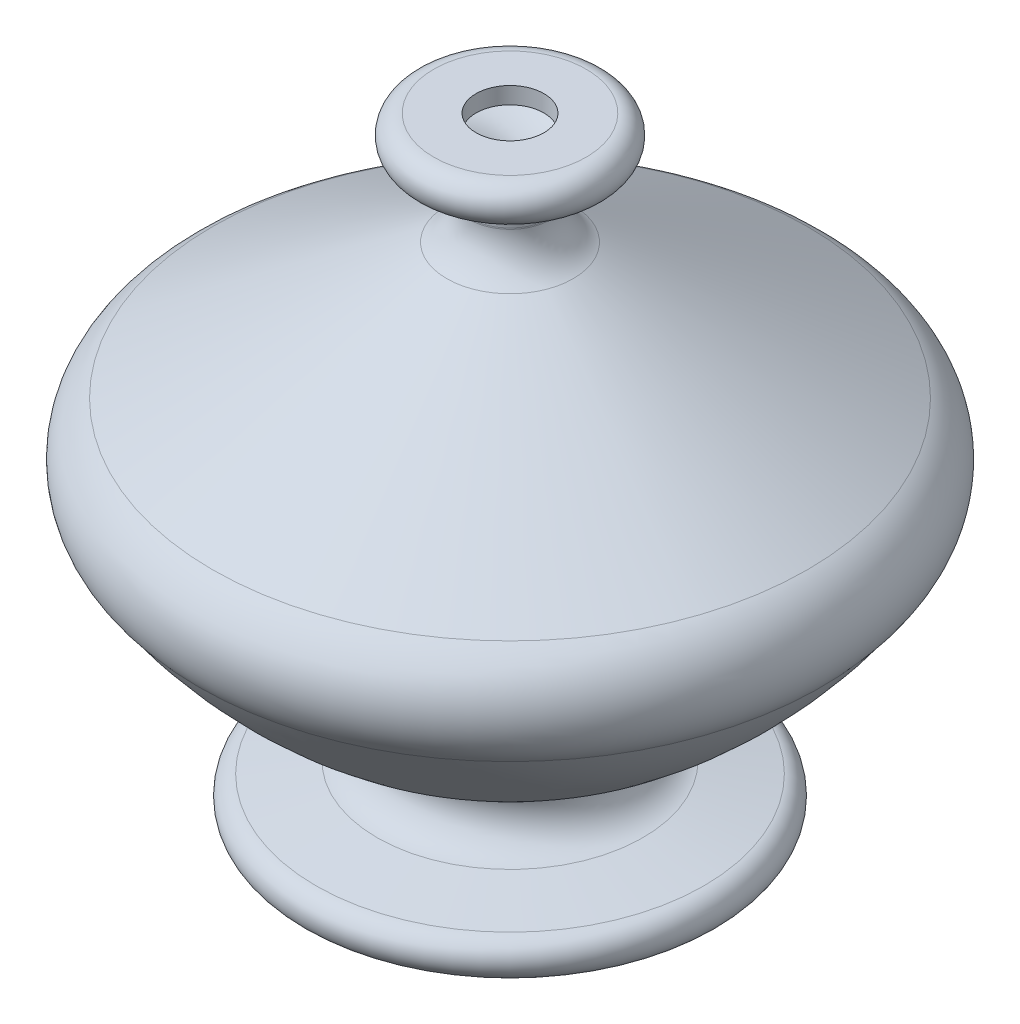
ISO-10303-21;
HEADER;
FILE_DESCRIPTION(('STEP AP214'),'2;1');
FILE_NAME('part.step','',(''),(''),'','','');
FILE_SCHEMA(('AUTOMOTIVE_DESIGN { 1 0 10303 214 1 1 1 1 }'));
ENDSEC;
DATA;
#1=APPLICATION_CONTEXT('core data for automotive mechanical design processes');
#2=APPLICATION_PROTOCOL_DEFINITION('international standard','automotive_design',2000,#1);
#3=PRODUCT_CONTEXT('',#1,'mechanical');
#4=PRODUCT('Part','Part','',(#3));
#5=PRODUCT_RELATED_PRODUCT_CATEGORY('part','',(#4));
#6=PRODUCT_DEFINITION_FORMATION('','',#4);
#7=PRODUCT_DEFINITION_CONTEXT('part definition',#1,'design');
#8=PRODUCT_DEFINITION('design','',#6,#7);
#9=PRODUCT_DEFINITION_SHAPE('','',#8);
#10=(LENGTH_UNIT() NAMED_UNIT(*) SI_UNIT(.MILLI.,.METRE.));
#11=(NAMED_UNIT(*) PLANE_ANGLE_UNIT() SI_UNIT($,.RADIAN.));
#12=(NAMED_UNIT(*) SI_UNIT($,.STERADIAN.) SOLID_ANGLE_UNIT());
#13=UNCERTAINTY_MEASURE_WITH_UNIT(LENGTH_MEASURE(1.E-05),#10,'distance_accuracy_value','');
#14=(GEOMETRIC_REPRESENTATION_CONTEXT(3) GLOBAL_UNCERTAINTY_ASSIGNED_CONTEXT((#13)) GLOBAL_UNIT_ASSIGNED_CONTEXT((#10,
#11,#12)) REPRESENTATION_CONTEXT('',''));
#15=CARTESIAN_POINT('',(0.,0.,0.));
#16=DIRECTION('',(0.,0.,1.));
#17=DIRECTION('',(1.,0.,0.));
#18=AXIS2_PLACEMENT_3D('',#15,#16,#17);
#19=CARTESIAN_POINT('',(0.,4.4,0.));
#20=DIRECTION('',(0.,1.,0.));
#21=DIRECTION('',(0.,0.,1.));
#22=AXIS2_PLACEMENT_3D('',#19,#20,#21);
#23=PLANE('',#22);
#24=CARTESIAN_POINT('',(0.,4.39999999999999,0.));
#25=DIRECTION('',(0.,1.,0.));
#26=DIRECTION('',(0.,0.,1.));
#27=AXIS2_PLACEMENT_3D('',#24,#25,#26);
#28=CIRCLE('',#27,50.);
#29=CARTESIAN_POINT('',(0.,4.39999999999999,50.));
#30=VERTEX_POINT('',#29);
#31=EDGE_CURVE('E10',#30,#30,#28,.T.);
#32=ORIENTED_EDGE('',*,*,#31,.T.);
#33=EDGE_LOOP('',(#32));
#34=FACE_BOUND('',#33,.T.);
#35=ADVANCED_FACE('F40',(#34),#23,.T.);
#36=CARTESIAN_POINT('',(0.,4.99999999999999,0.));
#37=DIRECTION('',(0.,1.,0.));
#38=DIRECTION('',(0.,0.,1.));
#39=AXIS2_PLACEMENT_3D('',#36,#37,#38);
#40=TOROIDAL_SURFACE('',#39,50.,0.599999999999995);
#41=CARTESIAN_POINT('',(0.,5.59021831279544,0.));
#42=DIRECTION('',(0.,1.,0.));
#43=DIRECTION('',(0.,0.,1.));
#44=AXIS2_PLACEMENT_3D('',#41,#42,#43);
#45=CIRCLE('',#44,50.1078996906432);
#46=CARTESIAN_POINT('',(0.,5.59021831279544,50.1078996906432));
#47=VERTEX_POINT('',#46);
#48=EDGE_CURVE('E43',#47,#47,#45,.T.);
#49=ORIENTED_EDGE('',*,*,#48,.T.);
#50=EDGE_LOOP('',(#49));
#51=FACE_BOUND('',#50,.T.);
#52=ORIENTED_EDGE('',*,*,#31,.F.);
#53=EDGE_LOOP('',(#52));
#54=FACE_BOUND('',#53,.T.);
#55=ADVANCED_FACE('F133',(#51,#54),#40,.F.);
#56=CARTESIAN_POINT('',(0.,5.59021831279544,0.));
#57=DIRECTION('',(0.,-1.,0.));
#58=DIRECTION('',(0.,0.,-1.));
#59=AXIS2_PLACEMENT_3D('',#56,#57,#58);
#60=CONICAL_SURFACE('',#59,50.1078996906432,1.38997983116206);
#61=CARTESIAN_POINT('',(0.,8.5184576809019,0.));
#62=DIRECTION('',(0.,1.,0.));
#63=DIRECTION('',(0.,0.,1.));
#64=AXIS2_PLACEMENT_3D('',#61,#62,#63);
#65=CIRCLE('',#64,34.0902402423009);
#66=CARTESIAN_POINT('',(0.,8.5184576809019,34.0902402423009));
#67=VERTEX_POINT('',#66);
#68=EDGE_CURVE('E50',#67,#67,#65,.T.);
#69=ORIENTED_EDGE('',*,*,#68,.T.);
#70=EDGE_LOOP('',(#69));
#71=FACE_BOUND('',#70,.T.);
#72=ORIENTED_EDGE('',*,*,#48,.F.);
#73=EDGE_LOOP('',(#72));
#74=FACE_BOUND('',#73,.T.);
#75=ADVANCED_FACE('F137',(#71,#74),#60,.F.);
#76=CARTESIAN_POINT('',(0.,21.7,0.));
#77=DIRECTION('',(0.,1.,0.));
#78=DIRECTION('',(0.,0.,1.));
#79=AXIS2_PLACEMENT_3D('',#76,#77,#78);
#80=TOROIDAL_SURFACE('',#79,36.5,13.4);
#81=CARTESIAN_POINT('',(0.,35.0477430693787,0.));
#82=DIRECTION('',(0.,1.,0.));
#83=DIRECTION('',(0.,0.,1.));
#84=AXIS2_PLACEMENT_3D('',#81,#82,#83);
#85=CIRCLE('',#84,35.3177331291744);
#86=CARTESIAN_POINT('',(0.,35.0477430693787,35.3177331291744));
#87=VERTEX_POINT('',#86);
#88=EDGE_CURVE('E51',#87,#87,#85,.T.);
#89=ORIENTED_EDGE('',*,*,#88,.T.);
#90=EDGE_LOOP('',(#89));
#91=FACE_BOUND('',#90,.T.);
#92=ORIENTED_EDGE('',*,*,#68,.F.);
#93=EDGE_LOOP('',(#92));
#94=FACE_BOUND('',#93,.T.);
#95=ADVANCED_FACE('F141',(#91,#94),#80,.T.);
#96=CARTESIAN_POINT('',(0.,141.481035556189,0.));
#97=DIRECTION('',(0.,1.,0.));
#98=DIRECTION('',(0.,0.,1.));
#99=AXIS2_PLACEMENT_3D('',#96,#97,#98);
#100=DEGENERATE_TOROIDAL_SURFACE('',#99,20.968270907506,120.4,.F.);
#101=CARTESIAN_POINT('',(0.,73.1766344230635,0.));
#102=DIRECTION('',(0.,1.,0.));
#103=DIRECTION('',(0.,0.,1.));
#104=AXIS2_PLACEMENT_3D('',#101,#102,#103);
#105=CIRCLE('',#104,78.1814582189275);
#106=CARTESIAN_POINT('',(0.,73.1766344230635,78.1814582189275));
#107=VERTEX_POINT('',#106);
#108=EDGE_CURVE('E57',#107,#107,#105,.T.);
#109=ORIENTED_EDGE('',*,*,#108,.T.);
#110=EDGE_LOOP('',(#109));
#111=FACE_BOUND('',#110,.T.);
#112=ORIENTED_EDGE('',*,*,#88,.F.);
#113=EDGE_LOOP('',(#112));
#114=FACE_BOUND('',#113,.T.);
#115=ADVANCED_FACE('F147',(#111,#114),#100,.T.);
#116=CARTESIAN_POINT('',(0.,81.4,0.));
#117=DIRECTION('',(0.,1.,0.));
#118=DIRECTION('',(0.,0.,1.));
#119=AXIS2_PLACEMENT_3D('',#116,#117,#118);
#120=TOROIDAL_SURFACE('',#119,70.,11.6);
#121=CARTESIAN_POINT('',(0.,91.4458946838995,0.));
#122=DIRECTION('',(0.,1.,0.));
#123=DIRECTION('',(0.,0.,1.));
#124=AXIS2_PLACEMENT_3D('',#121,#122,#123);
#125=CIRCLE('',#124,75.8000000000001);
#126=CARTESIAN_POINT('',(0.,91.4458946838994,-75.8000000000001));
#127=VERTEX_POINT('',#126);
#128=EDGE_CURVE('E56',#127,#127,#125,.T.);
#129=ORIENTED_EDGE('',*,*,#128,.T.);
#130=EDGE_LOOP('',(#129));
#131=FACE_BOUND('',#130,.T.);
#132=ORIENTED_EDGE('',*,*,#108,.F.);
#133=EDGE_LOOP('',(#132));
#134=FACE_BOUND('',#133,.T.);
#135=ADVANCED_FACE('F152',(#131,#134),#120,.F.);
#136=CARTESIAN_POINT('',(0.,91.4458946838995,0.));
#137=DIRECTION('',(0.,-1.,0.));
#138=DIRECTION('',(0.,0.,-1.));
#139=AXIS2_PLACEMENT_3D('',#136,#137,#138);
#140=CONICAL_SURFACE('',#139,75.8000000000001,1.04719755119659);
#141=CARTESIAN_POINT('',(0.,126.895201212143,0.));
#142=DIRECTION('',(0.,1.,0.));
#143=DIRECTION('',(0.,0.,1.));
#144=AXIS2_PLACEMENT_3D('',#141,#142,#143);
#145=CIRCLE('',#144,14.3999999999999);
#146=CARTESIAN_POINT('',(0.,126.895201212143,-14.4));
#147=VERTEX_POINT('',#146);
#148=EDGE_CURVE('E65',#147,#147,#145,.T.);
#149=CARTESIAN_POINT('',(0.,126.895201212143,-14.4));
#150=CARTESIAN_POINT('',(0.,126.525937602474,-15.0395833333333));
#151=CARTESIAN_POINT('',(0.,126.156673992805,-15.6791666666666));
#152=CARTESIAN_POINT('',(0.,125.418146773466,-16.9583333333333));
#153=CARTESIAN_POINT('',(0.,125.048883163797,-17.5979166666666));
#154=CARTESIAN_POINT('',(0.,124.310355944459,-18.8770833333333));
#155=CARTESIAN_POINT('',(0.,123.941092334789,-19.5166666666666));
#156=CARTESIAN_POINT('',(0.,123.202565115451,-20.7958333333333));
#157=CARTESIAN_POINT('',(0.,122.833301505782,-21.4354166666666));
#158=CARTESIAN_POINT('',(0.,122.094774286443,-22.7145833333333));
#159=CARTESIAN_POINT('',(0.,121.725510676774,-23.3541666666666));
#160=CARTESIAN_POINT('',(0.,120.986983457436,-24.6333333333333));
#161=CARTESIAN_POINT('',(0.,120.617719847767,-25.2729166666666));
#162=CARTESIAN_POINT('',(0.,119.879192628428,-26.5520833333333));
#163=CARTESIAN_POINT('',(0.,119.509929018759,-27.1916666666666));
#164=CARTESIAN_POINT('',(0.,118.771401799421,-28.4708333333333));
#165=CARTESIAN_POINT('',(0.,118.402138189751,-29.1104166666666));
#166=CARTESIAN_POINT('',(0.,117.663610970413,-30.3895833333333));
#167=CARTESIAN_POINT('',(0.,117.294347360744,-31.0291666666666));
#168=CARTESIAN_POINT('',(0.,116.555820141405,-32.3083333333333));
#169=CARTESIAN_POINT('',(0.,116.186556531736,-32.9479166666667));
#170=CARTESIAN_POINT('',(0.,115.448029312398,-34.2270833333333));
#171=CARTESIAN_POINT('',(0.,115.078765702728,-34.8666666666667));
#172=CARTESIAN_POINT('',(0.,114.34023848339,-36.1458333333333));
#173=CARTESIAN_POINT('',(0.,113.970974873721,-36.7854166666667));
#174=CARTESIAN_POINT('',(0.,113.232447654382,-38.0645833333333));
#175=CARTESIAN_POINT('',(0.,112.863184044713,-38.7041666666667));
#176=CARTESIAN_POINT('',(0.,112.124656825375,-39.9833333333333));
#177=CARTESIAN_POINT('',(0.,111.755393215706,-40.6229166666667));
#178=CARTESIAN_POINT('',(0.,111.016865996367,-41.9020833333333));
#179=CARTESIAN_POINT('',(0.,110.647602386698,-42.5416666666667));
#180=CARTESIAN_POINT('',(0.,109.90907516736,-43.8208333333333));
#181=CARTESIAN_POINT('',(0.,109.53981155769,-44.4604166666667));
#182=CARTESIAN_POINT('',(0.,108.801284338352,-45.7395833333333));
#183=CARTESIAN_POINT('',(0.,108.432020728683,-46.3791666666667));
#184=CARTESIAN_POINT('',(0.,107.693493509344,-47.6583333333333));
#185=CARTESIAN_POINT('',(0.,107.324229899675,-48.2979166666667));
#186=CARTESIAN_POINT('',(0.,106.585702680337,-49.5770833333333));
#187=CARTESIAN_POINT('',(0.,106.216439070668,-50.2166666666667));
#188=CARTESIAN_POINT('',(0.,105.477911851329,-51.4958333333334));
#189=CARTESIAN_POINT('',(0.,105.10864824166,-52.1354166666667));
#190=CARTESIAN_POINT('',(0.,104.370121022322,-53.4145833333334));
#191=CARTESIAN_POINT('',(0.,104.000857412652,-54.0541666666667));
#192=CARTESIAN_POINT('',(0.,103.262330193314,-55.3333333333334));
#193=CARTESIAN_POINT('',(0.,102.893066583645,-55.9729166666667));
#194=CARTESIAN_POINT('',(0.,102.154539364306,-57.2520833333334));
#195=CARTESIAN_POINT('',(0.,101.785275754637,-57.8916666666667));
#196=CARTESIAN_POINT('',(0.,101.046748535299,-59.1708333333334));
#197=CARTESIAN_POINT('',(0.,100.67748492563,-59.8104166666667));
#198=CARTESIAN_POINT('',(0.,99.9389577062911,-61.0895833333334));
#199=CARTESIAN_POINT('',(0.,99.5696940966219,-61.7291666666667));
#200=CARTESIAN_POINT('',(0.,98.8311668772835,-63.0083333333334));
#201=CARTESIAN_POINT('',(0.,98.4619032676143,-63.6479166666667));
#202=CARTESIAN_POINT('',(0.,97.7233760482759,-64.9270833333334));
#203=CARTESIAN_POINT('',(0.,97.3541124386067,-65.5666666666667));
#204=CARTESIAN_POINT('',(0.,96.6155852192683,-66.8458333333334));
#205=CARTESIAN_POINT('',(0.,96.2463216095991,-67.4854166666667));
#206=CARTESIAN_POINT('',(0.,95.5077943902607,-68.7645833333334));
#207=CARTESIAN_POINT('',(0.,95.1385307805915,-69.4041666666667));
#208=CARTESIAN_POINT('',(0.,94.4000035612531,-70.6833333333334));
#209=CARTESIAN_POINT('',(0.,94.0307399515839,-71.3229166666667));
#210=CARTESIAN_POINT('',(0.,93.2922127322455,-72.6020833333334));
#211=CARTESIAN_POINT('',(0.,92.9229491225762,-73.2416666666667));
#212=CARTESIAN_POINT('',(0.,92.1844219032378,-74.5208333333334));
#213=CARTESIAN_POINT('',(0.,91.8151582935686,-75.1604166666667));
#214=CARTESIAN_POINT('',(0.,91.4458946838994,-75.8000000000001));
#215=B_SPLINE_CURVE_WITH_KNOTS('',3,(#149,#150,#151,#152,#153,#154,#155,#156,#157,#158,#159,
#160,#161,#162,#163,#164,#165,#166,#167,#168,#169,#170,#171,#172,#173,#174,#175,#176,#177,#178,
#179,#180,#181,#182,#183,#184,#185,#186,#187,#188,#189,#190,#191,#192,#193,#194,#195,#196,#197,
#198,#199,#200,#201,#202,#203,#204,#205,#206,#207,#208,#209,#210,#211,#212,#213,#214),
.UNSPECIFIED.,.F.,.F.,(4,2,2,2,2,2,2,2,2,2,2,2,2,2,2,2,2,2,2,2,2,2,2,2,2,2,2,2,2,2,2,2,4),(0.,
2.21558165801521,4.43116331603041,6.64674497404561,8.86232663206081,11.077908290076,
13.2934899480912,15.5090716061064,17.7246532641216,19.9402349221368,22.155816580152,
24.3713982381672,26.5869798961824,28.8025615541976,31.0181432122128,33.233724870228,
35.4493065282432,37.6648881862584,39.8804698442736,42.0960515022888,44.311633160304,
46.5272148183192,48.7427964763344,50.9583781343496,53.1739597923648,55.38954145038,
57.6051231083952,59.8207047664104,62.0362864244256,64.2518680824408,66.467449740456,
68.6830313984712,70.8986130564864),.UNSPECIFIED.);
#216=EDGE_CURVE('BSEAM158',#147,#127,#215,.T.);
#217=ORIENTED_EDGE('',*,*,#148,.T.);
#218=ORIENTED_EDGE('',*,*,#128,.F.);
#219=ORIENTED_EDGE('',*,*,#216,.T.);
#220=ORIENTED_EDGE('',*,*,#216,.F.);
#221=EDGE_LOOP('',(#217,#219,#218,#220));
#222=FACE_BOUND('',#221,.T.);
#223=ADVANCED_FACE('F158',(#222),#140,.F.);
#224=CARTESIAN_POINT('',(0.,141.098017834208,0.));
#225=DIRECTION('',(0.,1.,0.));
#226=DIRECTION('',(0.,0.,1.));
#227=AXIS2_PLACEMENT_3D('',#224,#225,#226);
#228=TOROIDAL_SURFACE('',#227,22.6,16.4);
#229=CARTESIAN_POINT('',(0.,141.098017834208,0.));
#230=DIRECTION('',(0.,1.,0.));
#231=DIRECTION('',(0.,0.,1.));
#232=AXIS2_PLACEMENT_3D('',#229,#230,#231);
#233=CIRCLE('',#232,6.2);
#234=CARTESIAN_POINT('',(0.,141.098017834208,6.2));
#235=VERTEX_POINT('',#234);
#236=EDGE_CURVE('E63',#235,#235,#233,.T.);
#237=ORIENTED_EDGE('',*,*,#236,.T.);
#238=EDGE_LOOP('',(#237));
#239=FACE_BOUND('',#238,.T.);
#240=ORIENTED_EDGE('',*,*,#148,.F.);
#241=EDGE_LOOP('',(#240));
#242=FACE_BOUND('',#241,.T.);
#243=ADVANCED_FACE('F165',(#239,#242),#228,.T.);
#244=CARTESIAN_POINT('',(0.,194.540686073728,0.));
#245=DIRECTION('',(0.,1.,0.));
#246=DIRECTION('',(0.,0.,1.));
#247=AXIS2_PLACEMENT_3D('',#244,#245,#246);
#248=CYLINDRICAL_SURFACE('',#247,6.2);
#249=CARTESIAN_POINT('',(0.,141.403935941769,0.));
#250=DIRECTION('',(0.,1.,0.));
#251=DIRECTION('',(0.,0.,1.));
#252=AXIS2_PLACEMENT_3D('',#249,#250,#251);
#253=CIRCLE('',#252,6.19999999999999);
#254=CARTESIAN_POINT('',(0.,141.403935941769,6.19999999999999));
#255=VERTEX_POINT('',#254);
#256=EDGE_CURVE('E68',#255,#255,#253,.T.);
#257=ORIENTED_EDGE('',*,*,#256,.T.);
#258=EDGE_LOOP('',(#257));
#259=FACE_BOUND('',#258,.T.);
#260=ORIENTED_EDGE('',*,*,#236,.F.);
#261=EDGE_LOOP('',(#260));
#262=FACE_BOUND('',#261,.T.);
#263=ADVANCED_FACE('F167',(#259,#262),#248,.F.);
#264=CARTESIAN_POINT('',(0.,141.403935941769,0.));
#265=DIRECTION('',(0.,1.,0.));
#266=DIRECTION('',(0.,0.,1.));
#267=AXIS2_PLACEMENT_3D('',#264,#265,#266);
#268=TOROIDAL_SURFACE('',#267,18.6,12.4);
#269=CARTESIAN_POINT('',(0.,153.5281168675,0.));
#270=DIRECTION('',(0.,1.,0.));
#271=DIRECTION('',(0.,0.,1.));
#272=AXIS2_PLACEMENT_3D('',#269,#270,#271);
#273=CIRCLE('',#272,15.9991853429861);
#274=CARTESIAN_POINT('',(0.,153.5281168675,15.9991853429861));
#275=VERTEX_POINT('',#274);
#276=EDGE_CURVE('E72',#275,#275,#273,.T.);
#277=ORIENTED_EDGE('',*,*,#276,.T.);
#278=EDGE_LOOP('',(#277));
#279=FACE_BOUND('',#278,.T.);
#280=ORIENTED_EDGE('',*,*,#256,.F.);
#281=EDGE_LOOP('',(#280));
#282=FACE_BOUND('',#281,.T.);
#283=ADVANCED_FACE('F168',(#279,#282),#268,.T.);
#284=CARTESIAN_POINT('',(0.,153.5281168675,0.));
#285=DIRECTION('',(0.,1.,0.));
#286=DIRECTION('',(0.,0.,1.));
#287=AXIS2_PLACEMENT_3D('',#284,#285,#286);
#288=CONICAL_SURFACE('',#287,15.9991853429861,1.35948410089142);
#289=CARTESIAN_POINT('',(0.,154.413346084239,0.));
#290=DIRECTION('',(0.,1.,0.));
#291=DIRECTION('',(0.,0.,1.));
#292=AXIS2_PLACEMENT_3D('',#289,#290,#291);
#293=CIRCLE('',#292,20.1258458705007);
#294=CARTESIAN_POINT('',(0.,154.413346084239,20.1258458705007));
#295=VERTEX_POINT('',#294);
#296=EDGE_CURVE('E74',#295,#295,#293,.T.);
#297=ORIENTED_EDGE('',*,*,#296,.T.);
#298=EDGE_LOOP('',(#297));
#299=FACE_BOUND('',#298,.T.);
#300=ORIENTED_EDGE('',*,*,#276,.F.);
#301=EDGE_LOOP('',(#300));
#302=FACE_BOUND('',#301,.T.);
#303=ADVANCED_FACE('F171',(#299,#302),#288,.F.);
#304=CARTESIAN_POINT('',(0.,155.,0.));
#305=DIRECTION('',(0.,1.,0.));
#306=DIRECTION('',(0.,0.,1.));
#307=AXIS2_PLACEMENT_3D('',#304,#305,#306);
#308=TOROIDAL_SURFACE('',#307,20.,0.599999999999995);
#309=CARTESIAN_POINT('',(0.,155.6,0.));
#310=DIRECTION('',(0.,1.,0.));
#311=DIRECTION('',(0.,0.,1.));
#312=AXIS2_PLACEMENT_3D('',#309,#310,#311);
#313=CIRCLE('',#312,20.);
#314=CARTESIAN_POINT('',(0.,155.6,20.));
#315=VERTEX_POINT('',#314);
#316=EDGE_CURVE('E80',#315,#315,#313,.T.);
#317=ORIENTED_EDGE('',*,*,#316,.T.);
#318=EDGE_LOOP('',(#317));
#319=FACE_BOUND('',#318,.T.);
#320=ORIENTED_EDGE('',*,*,#296,.F.);
#321=EDGE_LOOP('',(#320));
#322=FACE_BOUND('',#321,.T.);
#323=ADVANCED_FACE('F178',(#319,#322),#308,.F.);
#324=CARTESIAN_POINT('',(-20.,155.6,0.));
#325=DIRECTION('',(0.,-1.,0.));
#326=DIRECTION('',(0.,0.,-1.));
#327=AXIS2_PLACEMENT_3D('',#324,#325,#326);
#328=PLANE('',#327);
#329=CARTESIAN_POINT('',(0.,155.6,0.));
#330=DIRECTION('',(0.,1.,0.));
#331=DIRECTION('',(0.,0.,1.));
#332=AXIS2_PLACEMENT_3D('',#329,#330,#331);
#333=CIRCLE('',#332,8.9);
#334=CARTESIAN_POINT('',(0.,155.6,8.9));
#335=VERTEX_POINT('',#334);
#336=EDGE_CURVE('E78',#335,#335,#333,.T.);
#337=ORIENTED_EDGE('',*,*,#336,.T.);
#338=EDGE_LOOP('',(#337));
#339=FACE_BOUND('',#338,.T.);
#340=ORIENTED_EDGE('',*,*,#316,.F.);
#341=EDGE_LOOP('',(#340));
#342=FACE_BOUND('',#341,.T.);
#343=ADVANCED_FACE('F185',(#339,#342),#328,.T.);
#344=CARTESIAN_POINT('',(0.,194.540686073728,0.));
#345=DIRECTION('',(0.,1.,0.));
#346=DIRECTION('',(0.,0.,1.));
#347=AXIS2_PLACEMENT_3D('',#344,#345,#346);
#348=CYLINDRICAL_SURFACE('',#347,8.9);
#349=CARTESIAN_POINT('',(0.,160.,0.));
#350=DIRECTION('',(0.,1.,0.));
#351=DIRECTION('',(0.,0.,1.));
#352=AXIS2_PLACEMENT_3D('',#349,#350,#351);
#353=CIRCLE('',#352,8.9);
#354=CARTESIAN_POINT('',(0.,160.,8.9));
#355=VERTEX_POINT('',#354);
#356=EDGE_CURVE('E83',#355,#355,#353,.T.);
#357=ORIENTED_EDGE('',*,*,#356,.T.);
#358=EDGE_LOOP('',(#357));
#359=FACE_BOUND('',#358,.T.);
#360=ORIENTED_EDGE('',*,*,#336,.F.);
#361=EDGE_LOOP('',(#360));
#362=FACE_BOUND('',#361,.T.);
#363=ADVANCED_FACE('F187',(#359,#362),#348,.F.);
#364=CARTESIAN_POINT('',(-20.,160.,0.));
#365=DIRECTION('',(0.,1.,0.));
#366=DIRECTION('',(0.,0.,1.));
#367=AXIS2_PLACEMENT_3D('',#364,#365,#366);
#368=PLANE('',#367);
#369=CARTESIAN_POINT('',(0.,160.,0.));
#370=DIRECTION('',(0.,1.,0.));
#371=DIRECTION('',(0.,0.,1.));
#372=AXIS2_PLACEMENT_3D('',#369,#370,#371);
#373=CIRCLE('',#372,20.);
#374=CARTESIAN_POINT('',(0.,160.,20.));
#375=VERTEX_POINT('',#374);
#376=EDGE_CURVE('E88',#375,#375,#373,.T.);
#377=ORIENTED_EDGE('',*,*,#376,.T.);
#378=EDGE_LOOP('',(#377));
#379=FACE_BOUND('',#378,.T.);
#380=ORIENTED_EDGE('',*,*,#356,.F.);
#381=EDGE_LOOP('',(#380));
#382=FACE_BOUND('',#381,.T.);
#383=ADVANCED_FACE('F188',(#379,#382),#368,.T.);
#384=CARTESIAN_POINT('',(0.,155.,0.));
#385=DIRECTION('',(0.,1.,0.));
#386=DIRECTION('',(0.,0.,1.));
#387=AXIS2_PLACEMENT_3D('',#384,#385,#386);
#388=TOROIDAL_SURFACE('',#387,20.,4.99999999999999);
#389=CARTESIAN_POINT('',(0.,150.111217368657,0.));
#390=DIRECTION('',(0.,1.,0.));
#391=DIRECTION('',(0.,0.,1.));
#392=AXIS2_PLACEMENT_3D('',#389,#390,#391);
#393=CIRCLE('',#392,21.0487155875056);
#394=CARTESIAN_POINT('',(0.,150.111217368657,21.0487155875056));
#395=VERTEX_POINT('',#394);
#396=EDGE_CURVE('E90',#395,#395,#393,.T.);
#397=ORIENTED_EDGE('',*,*,#396,.T.);
#398=EDGE_LOOP('',(#397));
#399=FACE_BOUND('',#398,.T.);
#400=ORIENTED_EDGE('',*,*,#376,.F.);
#401=EDGE_LOOP('',(#400));
#402=FACE_BOUND('',#401,.T.);
#403=ADVANCED_FACE('F192',(#399,#402),#388,.T.);
#404=CARTESIAN_POINT('',(0.,150.111217368657,0.));
#405=DIRECTION('',(0.,1.,0.));
#406=DIRECTION('',(0.,0.,1.));
#407=AXIS2_PLACEMENT_3D('',#404,#405,#406);
#408=CONICAL_SURFACE('',#407,21.0487155875056,1.35948410089141);
#409=CARTESIAN_POINT('',(0.,149.225988151918,0.));
#410=DIRECTION('',(0.,1.,0.));
#411=DIRECTION('',(0.,0.,1.));
#412=AXIS2_PLACEMENT_3D('',#409,#410,#411);
#413=CIRCLE('',#412,16.922055059991);
#414=CARTESIAN_POINT('',(0.,149.225988151918,16.922055059991));
#415=VERTEX_POINT('',#414);
#416=EDGE_CURVE('E95',#415,#415,#413,.T.);
#417=ORIENTED_EDGE('',*,*,#416,.T.);
#418=EDGE_LOOP('',(#417));
#419=FACE_BOUND('',#418,.T.);
#420=ORIENTED_EDGE('',*,*,#396,.F.);
#421=EDGE_LOOP('',(#420));
#422=FACE_BOUND('',#421,.T.);
#423=ADVANCED_FACE('F196',(#419,#422),#408,.T.);
#424=CARTESIAN_POINT('',(0.,141.403935941769,0.));
#425=DIRECTION('',(0.,1.,0.));
#426=DIRECTION('',(0.,0.,1.));
#427=AXIS2_PLACEMENT_3D('',#424,#425,#426);
#428=TOROIDAL_SURFACE('',#427,18.6,8.00000000000001);
#429=CARTESIAN_POINT('',(0.,141.403935941769,0.));
#430=DIRECTION('',(0.,1.,0.));
#431=DIRECTION('',(0.,0.,1.));
#432=AXIS2_PLACEMENT_3D('',#429,#430,#431);
#433=CIRCLE('',#432,10.6);
#434=CARTESIAN_POINT('',(0.,141.403935941769,10.6));
#435=VERTEX_POINT('',#434);
#436=EDGE_CURVE('E92',#435,#435,#433,.T.);
#437=ORIENTED_EDGE('',*,*,#436,.T.);
#438=EDGE_LOOP('',(#437));
#439=FACE_BOUND('',#438,.T.);
#440=ORIENTED_EDGE('',*,*,#416,.F.);
#441=EDGE_LOOP('',(#440));
#442=FACE_BOUND('',#441,.T.);
#443=ADVANCED_FACE('F205',(#439,#442),#428,.F.);
#444=CARTESIAN_POINT('',(0.,194.540686073728,0.));
#445=DIRECTION('',(0.,1.,0.));
#446=DIRECTION('',(0.,0.,1.));
#447=AXIS2_PLACEMENT_3D('',#444,#445,#446);
#448=CYLINDRICAL_SURFACE('',#447,10.6);
#449=CARTESIAN_POINT('',(0.,141.098017834208,0.));
#450=DIRECTION('',(0.,1.,0.));
#451=DIRECTION('',(0.,0.,1.));
#452=AXIS2_PLACEMENT_3D('',#449,#450,#451);
#453=CIRCLE('',#452,10.6);
#454=CARTESIAN_POINT('',(0.,141.098017834208,10.6));
#455=VERTEX_POINT('',#454);
#456=EDGE_CURVE('E98',#455,#455,#453,.T.);
#457=ORIENTED_EDGE('',*,*,#456,.T.);
#458=EDGE_LOOP('',(#457));
#459=FACE_BOUND('',#458,.T.);
#460=ORIENTED_EDGE('',*,*,#436,.F.);
#461=EDGE_LOOP('',(#460));
#462=FACE_BOUND('',#461,.T.);
#463=ADVANCED_FACE('F206',(#459,#462),#448,.T.);
#464=CARTESIAN_POINT('',(0.,141.098017834208,0.));
#465=DIRECTION('',(0.,1.,0.));
#466=DIRECTION('',(0.,0.,1.));
#467=AXIS2_PLACEMENT_3D('',#464,#465,#466);
#468=TOROIDAL_SURFACE('',#467,22.6,12.);
#469=CARTESIAN_POINT('',(0.,130.705712988794,0.));
#470=DIRECTION('',(0.,1.,0.));
#471=DIRECTION('',(0.,0.,1.));
#472=AXIS2_PLACEMENT_3D('',#469,#470,#471);
#473=CIRCLE('',#472,16.5999999999999);
#474=CARTESIAN_POINT('',(0.,130.705712988794,-16.6));
#475=VERTEX_POINT('',#474);
#476=EDGE_CURVE('E101',#475,#475,#473,.T.);
#477=ORIENTED_EDGE('',*,*,#476,.T.);
#478=EDGE_LOOP('',(#477));
#479=FACE_BOUND('',#478,.T.);
#480=ORIENTED_EDGE('',*,*,#456,.F.);
#481=EDGE_LOOP('',(#480));
#482=FACE_BOUND('',#481,.T.);
#483=ADVANCED_FACE('F209',(#479,#482),#468,.F.);
#484=CARTESIAN_POINT('',(0.,130.705712988794,0.));
#485=DIRECTION('',(0.,-1.,0.));
#486=DIRECTION('',(0.,0.,-1.));
#487=AXIS2_PLACEMENT_3D('',#484,#485,#486);
#488=CONICAL_SURFACE('',#487,16.5999999999999,1.04719755119659);
#489=CARTESIAN_POINT('',(0.,95.256406460551,0.));
#490=DIRECTION('',(0.,1.,0.));
#491=DIRECTION('',(0.,0.,1.));
#492=AXIS2_PLACEMENT_3D('',#489,#490,#491);
#493=CIRCLE('',#492,78.0000000000001);
#494=CARTESIAN_POINT('',(0.,95.256406460551,-78.0000000000001));
#495=VERTEX_POINT('',#494);
#496=EDGE_CURVE('E102',#495,#495,#493,.T.);
#497=CARTESIAN_POINT('',(0.,95.256406460551,-78.0000000000001));
#498=CARTESIAN_POINT('',(0.,95.6256700702202,-77.3604166666667));
#499=CARTESIAN_POINT('',(0.,95.9949336798894,-76.7208333333334));
#500=CARTESIAN_POINT('',(0.,96.7334608992278,-75.4416666666667));
#501=CARTESIAN_POINT('',(0.,97.102724508897,-74.8020833333334));
#502=CARTESIAN_POINT('',(0.,97.8412517282354,-73.5229166666667));
#503=CARTESIAN_POINT('',(0.,98.2105153379046,-72.8833333333334));
#504=CARTESIAN_POINT('',(0.,98.949042557243,-71.6041666666667));
#505=CARTESIAN_POINT('',(0.,99.3183061669122,-70.9645833333334));
#506=CARTESIAN_POINT('',(0.,100.056833386251,-69.6854166666667));
#507=CARTESIAN_POINT('',(0.,100.42609699592,-69.0458333333334));
#508=CARTESIAN_POINT('',(0.,101.164624215258,-67.7666666666667));
#509=CARTESIAN_POINT('',(0.,101.533887824927,-67.1270833333334));
#510=CARTESIAN_POINT('',(0.,102.272415044266,-65.8479166666667));
#511=CARTESIAN_POINT('',(0.,102.641678653935,-65.2083333333334));
#512=CARTESIAN_POINT('',(0.,103.380205873273,-63.9291666666667));
#513=CARTESIAN_POINT('',(0.,103.749469482943,-63.2895833333334));
#514=CARTESIAN_POINT('',(0.,104.487996702281,-62.0104166666667));
#515=CARTESIAN_POINT('',(0.,104.85726031195,-61.3708333333334));
#516=CARTESIAN_POINT('',(0.,105.595787531289,-60.0916666666667));
#517=CARTESIAN_POINT('',(0.,105.965051140958,-59.4520833333334));
#518=CARTESIAN_POINT('',(0.,106.703578360296,-58.1729166666667));
#519=CARTESIAN_POINT('',(0.,107.072841969965,-57.5333333333334));
#520=CARTESIAN_POINT('',(0.,107.811369189304,-56.2541666666667));
#521=CARTESIAN_POINT('',(0.,108.180632798973,-55.6145833333334));
#522=CARTESIAN_POINT('',(0.,108.919160018311,-54.3354166666667));
#523=CARTESIAN_POINT('',(0.,109.288423627981,-53.6958333333334));
#524=CARTESIAN_POINT('',(0.,110.026950847319,-52.4166666666667));
#525=CARTESIAN_POINT('',(0.,110.396214456988,-51.7770833333334));
#526=CARTESIAN_POINT('',(0.,111.134741676327,-50.4979166666667));
#527=CARTESIAN_POINT('',(0.,111.504005285996,-49.8583333333334));
#528=CARTESIAN_POINT('',(0.,112.242532505334,-48.5791666666667));
#529=CARTESIAN_POINT('',(0.,112.611796115004,-47.9395833333334));
#530=CARTESIAN_POINT('',(0.,113.350323334342,-46.6604166666667));
#531=CARTESIAN_POINT('',(0.,113.719586944011,-46.0208333333333));
#532=CARTESIAN_POINT('',(0.,114.45811416335,-44.7416666666667));
#533=CARTESIAN_POINT('',(0.,114.827377773019,-44.1020833333333));
#534=CARTESIAN_POINT('',(0.,115.565904992357,-42.8229166666667));
#535=CARTESIAN_POINT('',(0.,115.935168602026,-42.1833333333334));
#536=CARTESIAN_POINT('',(0.,116.673695821365,-40.9041666666667));
#537=CARTESIAN_POINT('',(0.,117.042959431034,-40.2645833333333));
#538=CARTESIAN_POINT('',(0.,117.781486650372,-38.9854166666667));
#539=CARTESIAN_POINT('',(0.,118.150750260042,-38.3458333333333));
#540=CARTESIAN_POINT('',(0.,118.88927747938,-37.0666666666667));
#541=CARTESIAN_POINT('',(0.,119.258541089049,-36.4270833333333));
#542=CARTESIAN_POINT('',(0.,119.997068308388,-35.1479166666667));
#543=CARTESIAN_POINT('',(0.,120.366331918057,-34.5083333333333));
#544=CARTESIAN_POINT('',(0.,121.104859137395,-33.2291666666667));
#545=CARTESIAN_POINT('',(0.,121.474122747064,-32.5895833333333));
#546=CARTESIAN_POINT('',(0.,122.212649966403,-31.3104166666667));
#547=CARTESIAN_POINT('',(0.,122.581913576072,-30.6708333333333));
#548=CARTESIAN_POINT('',(0.,123.32044079541,-29.3916666666667));
#549=CARTESIAN_POINT('',(0.,123.68970440508,-28.7520833333333));
#550=CARTESIAN_POINT('',(0.,124.428231624418,-27.4729166666667));
#551=CARTESIAN_POINT('',(0.,124.797495234087,-26.8333333333333));
#552=CARTESIAN_POINT('',(0.,125.536022453426,-25.5541666666667));
#553=CARTESIAN_POINT('',(0.,125.905286063095,-24.9145833333333));
#554=CARTESIAN_POINT('',(0.,126.643813282433,-23.6354166666667));
#555=CARTESIAN_POINT('',(0.,127.013076892102,-22.9958333333333));
#556=CARTESIAN_POINT('',(0.,127.751604111441,-21.7166666666667));
#557=CARTESIAN_POINT('',(0.,128.12086772111,-21.0770833333333));
#558=CARTESIAN_POINT('',(0.,128.859394940448,-19.7979166666666));
#559=CARTESIAN_POINT('',(0.,129.228658550118,-19.1583333333333));
#560=CARTESIAN_POINT('',(0.,129.967185769456,-17.8791666666667));
#561=CARTESIAN_POINT('',(0.,130.336449379125,-17.2395833333333));
#562=CARTESIAN_POINT('',(0.,130.705712988794,-16.6));
#563=B_SPLINE_CURVE_WITH_KNOTS('',3,(#497,#498,#499,#500,#501,#502,#503,#504,#505,#506,#507,
#508,#509,#510,#511,#512,#513,#514,#515,#516,#517,#518,#519,#520,#521,#522,#523,#524,#525,#526,
#527,#528,#529,#530,#531,#532,#533,#534,#535,#536,#537,#538,#539,#540,#541,#542,#543,#544,#545,
#546,#547,#548,#549,#550,#551,#552,#553,#554,#555,#556,#557,#558,#559,#560,#561,#562),
.UNSPECIFIED.,.F.,.F.,(4,2,2,2,2,2,2,2,2,2,2,2,2,2,2,2,2,2,2,2,2,2,2,2,2,2,2,2,2,2,2,2,4),(0.,
2.21558165801519,4.4311633160304,6.64674497404561,8.8623266320608,11.077908290076,
13.2934899480912,15.5090716061064,17.7246532641216,19.9402349221368,22.155816580152,
24.3713982381672,26.5869798961824,28.8025615541976,31.0181432122128,33.233724870228,
35.4493065282432,37.6648881862584,39.8804698442736,42.0960515022888,44.311633160304,
46.5272148183192,48.7427964763344,50.9583781343496,53.1739597923648,55.38954145038,
57.6051231083952,59.8207047664104,62.0362864244256,64.2518680824408,66.4674497404559,
68.6830313984712,70.8986130564864),.UNSPECIFIED.);
#564=EDGE_CURVE('BSEAM212',#495,#475,#563,.T.);
#565=ORIENTED_EDGE('',*,*,#496,.T.);
#566=ORIENTED_EDGE('',*,*,#476,.F.);
#567=ORIENTED_EDGE('',*,*,#564,.T.);
#568=ORIENTED_EDGE('',*,*,#564,.F.);
#569=EDGE_LOOP('',(#565,#567,#566,#568));
#570=FACE_BOUND('',#569,.T.);
#571=ADVANCED_FACE('F212',(#570),#488,.T.);
#572=CARTESIAN_POINT('',(0.,81.4,0.));
#573=DIRECTION('',(0.,1.,0.));
#574=DIRECTION('',(0.,0.,1.));
#575=AXIS2_PLACEMENT_3D('',#572,#573,#574);
#576=TOROIDAL_SURFACE('',#575,70.,16.);
#577=CARTESIAN_POINT('',(0.,70.3693272826405,0.));
#578=DIRECTION('',(0.,1.,0.));
#579=DIRECTION('',(0.,0.,1.));
#580=AXIS2_PLACEMENT_3D('',#577,#578,#579);
#581=CIRCLE('',#580,81.5898343129875);
#582=CARTESIAN_POINT('',(0.,70.3693272826405,81.5898343129875));
#583=VERTEX_POINT('',#582);
#584=EDGE_CURVE('E110',#583,#583,#581,.T.);
#585=ORIENTED_EDGE('',*,*,#584,.T.);
#586=EDGE_LOOP('',(#585));
#587=FACE_BOUND('',#586,.T.);
#588=ORIENTED_EDGE('',*,*,#496,.F.);
#589=EDGE_LOOP('',(#588));
#590=FACE_BOUND('',#589,.T.);
#591=ADVANCED_FACE('F217',(#587,#590),#576,.T.);
#592=CARTESIAN_POINT('',(0.,141.481035556189,0.));
#593=DIRECTION('',(0.,1.,0.));
#594=DIRECTION('',(0.,0.,1.));
#595=AXIS2_PLACEMENT_3D('',#592,#593,#594);
#596=DEGENERATE_TOROIDAL_SURFACE('',#595,20.968270907506,124.8,.F.);
#597=CARTESIAN_POINT('',(0.,30.7,0.));
#598=DIRECTION('',(0.,1.,0.));
#599=DIRECTION('',(0.,0.,1.));
#600=AXIS2_PLACEMENT_3D('',#597,#598,#599);
#601=CIRCLE('',#600,36.5);
#602=CARTESIAN_POINT('',(0.,30.7,36.5));
#603=VERTEX_POINT('',#602);
#604=EDGE_CURVE('E109',#603,#603,#601,.T.);
#605=ORIENTED_EDGE('',*,*,#604,.T.);
#606=EDGE_LOOP('',(#605));
#607=FACE_BOUND('',#606,.T.);
#608=ORIENTED_EDGE('',*,*,#584,.F.);
#609=EDGE_LOOP('',(#608));
#610=FACE_BOUND('',#609,.T.);
#611=ADVANCED_FACE('F225',(#607,#610),#596,.F.);
#612=CARTESIAN_POINT('',(0.,21.7,0.));
#613=DIRECTION('',(0.,1.,0.));
#614=DIRECTION('',(0.,0.,1.));
#615=AXIS2_PLACEMENT_3D('',#612,#613,#614);
#616=TOROIDAL_SURFACE('',#615,36.5,9.00000000000001);
#617=CARTESIAN_POINT('',(0.,12.8467253080684,0.));
#618=DIRECTION('',(0.,1.,0.));
#619=DIRECTION('',(0.,0.,1.));
#620=AXIS2_PLACEMENT_3D('',#617,#618,#619);
#621=CIRCLE('',#620,34.8815046403513);
#622=CARTESIAN_POINT('',(0.,12.8467253080684,34.8815046403513));
#623=VERTEX_POINT('',#622);
#624=EDGE_CURVE('E114',#623,#623,#621,.T.);
#625=ORIENTED_EDGE('',*,*,#624,.T.);
#626=EDGE_LOOP('',(#625));
#627=FACE_BOUND('',#626,.T.);
#628=ORIENTED_EDGE('',*,*,#604,.F.);
#629=EDGE_LOOP('',(#628));
#630=FACE_BOUND('',#629,.T.);
#631=ADVANCED_FACE('F227',(#627,#630),#616,.F.);
#632=CARTESIAN_POINT('',(0.,12.8467253080684,0.));
#633=DIRECTION('',(0.,-1.,0.));
#634=DIRECTION('',(0.,0.,-1.));
#635=AXIS2_PLACEMENT_3D('',#632,#633,#634);
#636=CONICAL_SURFACE('',#635,34.8815046403513,1.38997983116206);
#637=CARTESIAN_POINT('',(0.,9.91848593996197,0.));
#638=DIRECTION('',(0.,1.,0.));
#639=DIRECTION('',(0.,0.,1.));
#640=AXIS2_PLACEMENT_3D('',#637,#638,#639);
#641=CIRCLE('',#640,50.8991640886937);
#642=CARTESIAN_POINT('',(0.,9.91848593996197,50.8991640886937));
#643=VERTEX_POINT('',#642);
#644=EDGE_CURVE('E117',#643,#643,#641,.T.);
#645=ORIENTED_EDGE('',*,*,#644,.T.);
#646=EDGE_LOOP('',(#645));
#647=FACE_BOUND('',#646,.T.);
#648=ORIENTED_EDGE('',*,*,#624,.F.);
#649=EDGE_LOOP('',(#648));
#650=FACE_BOUND('',#649,.T.);
#651=ADVANCED_FACE('F135',(#647,#650),#636,.T.);
#652=CARTESIAN_POINT('',(0.,4.99999999999999,0.));
#653=DIRECTION('',(0.,1.,0.));
#654=DIRECTION('',(0.,0.,1.));
#655=AXIS2_PLACEMENT_3D('',#652,#653,#654);
#656=TOROIDAL_SURFACE('',#655,50.,5.);
#657=CARTESIAN_POINT('',(0.,0.,0.));
#658=DIRECTION('',(0.,1.,0.));
#659=DIRECTION('',(0.,0.,1.));
#660=AXIS2_PLACEMENT_3D('',#657,#658,#659);
#661=CIRCLE('',#660,50.);
#662=CARTESIAN_POINT('',(0.,0.,50.));
#663=VERTEX_POINT('',#662);
#664=EDGE_CURVE('E116',#663,#663,#661,.T.);
#665=ORIENTED_EDGE('',*,*,#664,.T.);
#666=EDGE_LOOP('',(#665));
#667=FACE_BOUND('',#666,.T.);
#668=ORIENTED_EDGE('',*,*,#644,.F.);
#669=EDGE_LOOP('',(#668));
#670=FACE_BOUND('',#669,.T.);
#671=ADVANCED_FACE('F123',(#667,#670),#656,.T.);
#672=CARTESIAN_POINT('',(0.,0.,0.));
#673=DIRECTION('',(0.,-1.,0.));
#674=DIRECTION('',(0.,0.,-1.));
#675=AXIS2_PLACEMENT_3D('',#672,#673,#674);
#676=PLANE('',#675);
#677=ORIENTED_EDGE('',*,*,#664,.F.);
#678=EDGE_LOOP('',(#677));
#679=FACE_BOUND('',#678,.T.);
#680=ADVANCED_FACE('F127',(#679),#676,.T.);
#681=CLOSED_SHELL('',(#35,#55,#75,#95,#115,#135,#223,#243,#263,#283,#303,#323,#343,#363,#383,
#403,#423,#443,#463,#483,#571,#591,#611,#631,#651,#671,#680));
#682=MANIFOLD_SOLID_BREP('B2',#681);
#683=ADVANCED_BREP_SHAPE_REPRESENTATION('',(#18,#682),#14);
#684=SHAPE_DEFINITION_REPRESENTATION(#9,#683);
ENDSEC;
END-ISO-10303-21;
